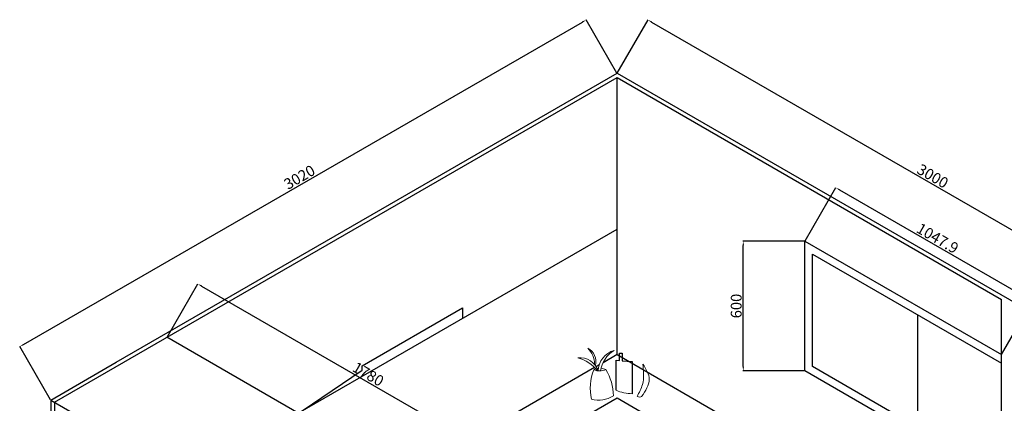
# Model space of a CAD drawing. Units: centimetres. Extents: x 209356 to 217348, y 253987 to 259034.
# Tile 5 of 7: x 209531 to 214078, y 257262 to 259034. Entities that reach past the tile are written whole.
import ezdxf

# ---------------------------------------------------------------- set-up
doc = ezdxf.new("R2010")
doc.units = ezdxf.units.CM
for name, color, linetype, lineweight in [('A-ANNO-DIMS', 2, 'Continuous', 18), ('A-ELEV', 7, 'Continuous', 25), ('A-FURN', 8, 'Continuous', 18)]:
    doc.layers.add(name, color=color, linetype=linetype, lineweight=lineweight)
doc.styles.get("Standard").update_dxf_attribs({"font": 'arial.ttf'})
doc.dimstyles.new('ISO-25', dxfattribs={"dimtxt": 50, "dimasz": 20, "dimexe": 1.25, "dimexo": 0.625, "dimtad": 1, "dimdec": 1, "dimtxsty": 'Standard', "dimcen": 2.5, "dimadec": 0, "dimazin": 0, "dimtfac": 1, "dimtdec": 1, "dimtmove": 0, "dimatfit": 3, "dimfxl": 1, "dimarcsym": 0})

# ---------------------------------------------------------------- blocks, each defined once
blk = doc.blocks.new('*D9')
at = {"layer": 'A-ANNO-DIMS', "color": 0, "lineweight": -2, "transparency": 16777216}
for p, q in [((209549, 257533.4), (212129.7, 259023.4)), ((212289.3, 258787.1), (212146.4, 259034.4)), ((209673.9, 257277.1), (209531, 257524.4))]:
    blk.add_line(p, q, dxfattribs=at)
at = {"layer": 'A-ANNO-DIMS', "color": 0, "transparency": 16777216}
for points in [[(212128.1, 259026.3), (212131.4, 259020.5), (212147.1, 259033.4)], [(209547.3, 257536.3), (209550.7, 257530.5), (209531.7, 257523.4)]]:
    blk.add_solid(points, dxfattribs=at)
at = {"layer": 'Defpoints', "color": 0, "transparency": 16777216}
for p in [(212147.1, 259033.4), (212289.6, 258786.5), (209674.2, 257276.5)]:
    blk.add_point(p, dxfattribs=at)
at = {"layer": 'A-ANNO-DIMS', "color": 0, "transparency": 16777216, "insert": (210826.3, 258301), "char_height": 50, "attachment_point": 5, "rotation": 30}
blk.add_mtext('3020', dxfattribs=at)
blk = doc.blocks.new('*D10')
at = {"layer": 'A-ANNO-DIMS', "color": 0, "lineweight": -2, "transparency": 16777216}
for p, q in [((212289.9, 258787.1), (212432.7, 259034.4)), ((212449.4, 259023.4), (215012.8, 257543.4)), ((214888, 257287.1), (215030.8, 257534.4))]:
    blk.add_line(p, q, dxfattribs=at)
at = {"layer": 'A-ANNO-DIMS', "color": 0, "transparency": 16777216}
for points in [[(212451.1, 259026.3), (212447.7, 259020.5), (212432.1, 259033.4)], [(215014.5, 257546.3), (215011.2, 257540.5), (215030.1, 257533.4)]]:
    blk.add_solid(points, dxfattribs=at)
at = {"layer": 'Defpoints', "color": 0, "transparency": 16777216}
for p in [(212289.6, 258786.5), (215030.1, 257533.4), (214887.6, 257286.5)]:
    blk.add_point(p, dxfattribs=at)
at = {"layer": 'A-ANNO-DIMS', "color": 0, "transparency": 16777216, "insert": (213744.2, 258306), "char_height": 50, "attachment_point": 5, "rotation": 330}
blk.add_mtext('3000', dxfattribs=at)
blk = doc.blocks.new('*D21')
at = {"layer": 'A-ANNO-DIMS', "color": 0, "lineweight": -2, "transparency": 16777216}
for p, q in [((213156.8, 258011.2), (212871.2, 258011.2)), ((212872.4, 257431.2), (212872.4, 257991.2)), ((213156.8, 257411.2), (212871.2, 257411.2))]:
    blk.add_line(p, q, dxfattribs=at)
at = {"layer": 'A-ANNO-DIMS', "color": 0, "transparency": 16777216}
for points in [[(212869.1, 257991.2), (212875.8, 257991.2), (212872.4, 258011.2)], [(212869.1, 257431.2), (212875.8, 257431.2), (212872.4, 257411.2)]]:
    blk.add_solid(points, dxfattribs=at)
at = {"layer": 'Defpoints', "color": 0, "transparency": 16777216}
for p in [(212872.4, 258011.2), (213157.4, 258011.2), (213157.4, 257411.2)]:
    blk.add_point(p, dxfattribs=at)
at = {"layer": 'A-ANNO-DIMS', "color": 0, "transparency": 16777216, "insert": (212846.3, 257711.2), "char_height": 50, "attachment_point": 5, "rotation": 90}
blk.add_mtext('600', dxfattribs=at)
blk = doc.blocks.new('*D22')
at = {"layer": 'A-ANNO-DIMS', "color": 0, "lineweight": -2, "transparency": 16777216}
for p, q in [((213157.7, 258011.7), (213300.5, 258259.1)), ((213317.2, 258248), (214190.1, 257744.1)), ((214065.2, 257487.8), (214208, 257735.2))]:
    blk.add_line(p, q, dxfattribs=at)
at = {"layer": 'A-ANNO-DIMS', "color": 0, "transparency": 16777216}
for points in [[(213318.9, 258250.9), (213315.6, 258245.1), (213299.9, 258258)], [(214191.8, 257747), (214188.4, 257741.2), (214207.4, 257734.1)]]:
    blk.add_solid(points, dxfattribs=at)
at = {"layer": 'Defpoints', "color": 0, "transparency": 16777216}
for p in [(213157.4, 258011.2), (214207.4, 257734.1), (214064.9, 257487.3)]:
    blk.add_point(p, dxfattribs=at)
at = {"layer": 'A-ANNO-DIMS', "color": 0, "transparency": 16777216, "insert": (213766.7, 258018.7), "char_height": 50, "attachment_point": 5, "rotation": 330}
blk.add_mtext('1047.9', dxfattribs=at)
blk = doc.blocks.new('*D35')
at = {"layer": 'A-ANNO-DIMS', "color": 0, "lineweight": -2, "transparency": 16777216}
for p, q in [((210211.4, 257567.1), (210354.2, 257814.4)), ((210370.9, 257803.4), (211877.8, 256933.4)), ((211752.9, 256677.1), (211895.8, 256924.4))]:
    blk.add_line(p, q, dxfattribs=at)
at = {"layer": 'A-ANNO-DIMS', "color": 0, "transparency": 16777216}
for points in [[(210372.6, 257806.3), (210369.3, 257800.5), (210353.6, 257813.4)], [(211879.5, 256936.3), (211876.1, 256930.5), (211895.1, 256923.4)]]:
    blk.add_solid(points, dxfattribs=at)
at = {"layer": 'Defpoints', "color": 0, "transparency": 16777216}
for p in [(210211.1, 257566.5), (211895.1, 256923.4), (211752.6, 256676.5)]:
    blk.add_point(p, dxfattribs=at)
at = {"layer": 'A-ANNO-DIMS', "color": 0, "transparency": 16777216, "insert": (211137.4, 257391), "char_height": 50, "attachment_point": 5, "rotation": 330}
blk.add_mtext('1780', dxfattribs=at)

msp = doc.modelspace()

# ---------------------------------------------------------------- linework, layer by layer
at = {"layer": 'A-ELEV'}
for p, q in [((209691.4926, 257266.5492), (212289.5688, 258766.5492)), ((209977.281, 257451.5492), (212289.5688, 258786.5492)), ((212289.5688, 258786.5492), (214887.645, 257286.5492)), ((212289.5688, 257486.5492), (212289.5688, 258766.5492)), ((212289.5688, 258766.5492), (214064.9209, 257741.5492)), ((210817.3256, 257216.5492), (212289.5688, 258066.5492)), ((213157.4217, 257411.1985), (213157.4217, 258011.1985)), ((213157.4217, 258011.1985), (214064.9209, 257487.2537)), ((213192.0627, 257951.1985), (214064.9209, 257447.2537)), ((213192.0627, 257431.1985), (213192.0627, 257951.1985)), ((214064.9209, 255341.5492), (214064.9209, 257741.5492)), ((211113.0858, 257435.2401), (211575.9368, 257702.4672)), ((211575.9368, 257702.4672), (211575.9368, 257654.5335)), ((213677.037, 257671.1985), (213677.037, 257151.1985)), ((211752.633, 256676.5492), (210211.1078, 257566.5492)), ((212300.5878, 257458.8151), (212300.5878, 257493.5451)), ((212300.5878, 257493.5451), (212312.9766, 257493.5451)), ((212312.9766, 257493.5451), (212312.9766, 257457.2872)), ((209674.1721, 257276.5492), (209977.281, 257451.5492)), ((212289.5688, 257486.5492), (212225.1361, 257449.3489)), ((212285.118, 257321.7061), (212285.118, 257460.7231)), ((212285.118, 257460.7231), (212300.5878, 257458.8151)), ((212289.5688, 257486.5492), (214064.9209, 256461.5492)), ((212312.9766, 257457.2872), (212359.43, 257455.5625)), ((212359.43, 257455.5625), (212359.43, 257305.5829)), ((210834.8943, 257226.6924), (211113.0858, 257415.2401)), ((211113.0858, 257415.2401), (211113.0858, 257435.2401)), ((212186.0099, 257426.7594), (211319.6203, 256926.5492)), ((212207.2514, 257439.0232), (212193.2219, 257430.9233)), ((214064.9209, 256887.2537), (213157.4217, 257411.1985)), ((214064.9209, 256927.2537), (213192.0627, 257431.1985)), ((209674.1721, 257276.5492), (209674.1721, 255776.5492)), ((209674.1721, 257276.5492), (211233.0178, 256376.5492)), ((209691.4926, 257266.5492), (209691.4926, 255786.5492)), ((211492.8254, 256826.5492), (212289.5688, 257286.5492)), ((212289.5688, 257286.5492), (214064.9209, 256261.5492))]:
    msp.add_line(p, q, dxfattribs=at)
at = {"layer": 'A-FURN'}
for centre, radius, start, end in [((212122.9519, 257454.8283), 69.0956, 344.5681144, 63.1670639), ((212087.3422, 257445.2494), 97.6548, 358.2525291, 46.8406578), ((212307.2765, 257405.6093), 105.4586, 107.1540601, 176.8459291), ((212349.7029, 257389.2204), 138.3196, 122.1135369, 170.8466772), ((212120.3433, 257386.4988), 85.3512, 16.9710223, 97.7873045), ((212069.1733, 257312.5536), 163.3823, 37.3987748, 75.9712723), ((212406.6187, 257331.4121), 240.63, 159.2149072, 192.2750133), ((212210.7038, 257359.414), 64.3246, 107.3357461, 116.8518427), ((212208.678, 257477.6976), 66.6236, 246.0655439, 295.8968662), ((212210.7038, 257359.414), 64.3246, 96.5964714, 101.6036326), ((212210.7038, 257359.414), 64.3246, 65.1105675, 85.5368305), ((212027.6969, 257290.7676), 245.482, 1.2053497, 31.153727), ((212370.5227, 257536.0246), 230.7085, 248.2730037, 267.2440909), ((212204.0986, 257406.1295), 130.0315, 255.4765971, 302.0622251)]:
    msp.add_arc(centre, radius, start, end, dxfattribs=at)
for points, knots in [([(212381.7931, 257293.1374), (212391.7606, 257311.2381), (212417.2191, 257357.4698), (212411.8955, 257410.6599), (212408.6562, 257443.0249)], [0, 0, 0, 0, 60.827228771, 155.360749571, 155.360749571, 155.360749571, 155.360749571]), ([(212408.6562, 257443.0249), (212423.34, 257419.289), (212454.5026, 257368.916), (212420.8533, 257319.3486), (212403.0597, 257293.1374)], [0, 0, 0, 0, 76.973267261, 163.355025742, 163.355025742, 163.355025742, 163.355025742]), ([(212381.7931, 257293.1374), (212390.0846, 257290.8691), (212400.8094, 257287.9352), (212405.4977, 257296.386), (212406.5613, 257298.3032)], [0, 0, 0, 0, 21.266589431, 27.507394445, 27.507394445, 27.507394445, 27.507394445])]:
    msp.add_open_spline(points, degree=3, knots=knots, dxfattribs=at)

# ---------------------------------------------------------------- dimensions: what is measured, and where the dimension line sits
at = {"layer": 'A-ANNO-DIMS'}
for base, p1, p2, angle, override, picture, middle in [((212147.0688, 259033.3664), (209674.1721, 257276.5492), (212289.5688, 258786.5492), 30, {"dimdec": 0, "dimlfac": 1, "dimrnd": 0, "dimzin": 0, "dimdsep": 46, "dimlunit": 2}, '*D9', (210826.2851, 258301.0309)), ((215030.145, 257533.3664), (212289.5688, 258786.5492), (214887.645, 257286.5492), 330, {"dimdec": 0, "dimlfac": 1, "dimrnd": 0, "dimzin": 0, "dimdsep": 46, "dimlunit": 2}, '*D10', (213744.1922, 258306.0309)), ((214207.4209, 257734.0709), (213157.4217, 258011.1985), (214064.9209, 257487.2537), 330, {"dimdec": 1, "dimlfac": 1, "dimrnd": 0, "dimzin": 0, "dimdsep": 46, "dimlunit": 2}, '*D22', (213766.7481, 258018.6931)), ((212872.4217, 258011.1985), (213157.4217, 257411.1985), (213157.4217, 258011.1985), 90, {"dimdec": 0, "dimlfac": 1, "dimrnd": 0, "dimzin": 0, "dimdsep": 46, "dimlunit": 2}, '*D21', (212846.2681, 257711.1985)), ((211895.133, 256923.3664), (210211.1078, 257566.5492), (211752.633, 256676.5492), 330, {"dimdec": 0, "dimlfac": 1, "dimrnd": 0, "dimzin": 0, "dimdsep": 46, "dimlunit": 2}, '*D35', (211137.4472, 257391.0161))]:
    dim = msp.add_linear_dim(base=base, p1=p1, p2=p2, angle=angle, dimstyle='ISO-25', override=override, dxfattribs=at)
    dim.commit()
    dim.dimension.update_dxf_attribs({"geometry": picture, "text_midpoint": middle})

doc.saveas('drawing.dxf')
